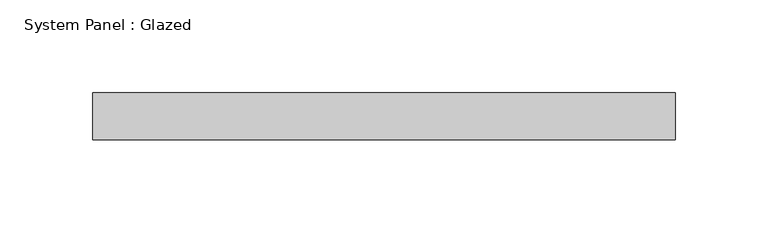
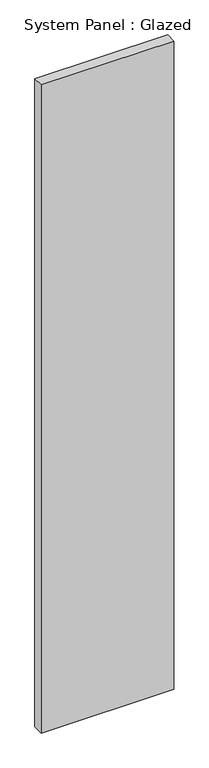
"""IFC4 building model written with IfcOpenShell, lengths in millimetres: plate geometry, System Panel : Glazed."""

from ifc_helpers import new_model, si_unit, origin, origin_with_axes, place, context, project, spatial, polyline, outline, extrude, source, transform, mapped, element, save


def system_panel_glazed_6d1bb68c(model_context):
    return source(origin(), model_context, "Body", "SweptSolid", [
        extrude(outline(polyline([(157.3561662, 19.05), (-157.3561662, 19.05), (-157.3561662, 44.45), (157.3561662, 44.45), (157.3561662, 19.05)])), origin_with_axes(), (0.0, 0.0, 1.0), 1625.6),
    ])


if __name__ == "__main__":
    model = new_model("IFC4")
    model_context = context("Model", 3, world=origin())
    ifc_project = project(units=[si_unit("LENGTHUNIT", "METRE", prefix="MILLI")], contexts=[model_context])
    site = spatial("IfcSite", under=ifc_project)
    building = spatial("IfcBuilding", under=site)
    placement = place(None, origin())
    system_panel_glazed_shape = system_panel_glazed_6d1bb68c(model_context)
    element("IfcPlate", 1, ObjectType="System Panel : Glazed", at=placement, inside=building, context=model_context, shape_type="MappedRepresentation", body=[
        mapped(system_panel_glazed_shape, transform((0.0, 0.0, 0.0), x_axis=(1.0, 0.0, 0.0), y_axis=(0.0, 1.0, 0.0), z_axis=(0.0, 0.0, 1.0))),
    ])
    save(model, "model.ifc")

# Revit data of these elements
# Type "System Panel : Glazed"
#   Construction Type Id = "GSP4R"
#   Analytic Construction = "1/8 in Pilkington single glazing"
#   Visual Light Transmittance = 0.9
#   Solar Heat Gain Coefficient = 0.86
#   Heat Transfer Coefficient (U) = 1.18115 BTU/(h·ft²·°F)
# Element 1 (IfcPlate, "System Panel : Glazed")
#   Materials on its faces: "Glass"
# Materials
#   "Glass": class "Glass", colour RGB 0 128 192, transparency 0.75, Description = "Soda Lime Glass", Cost = 0
